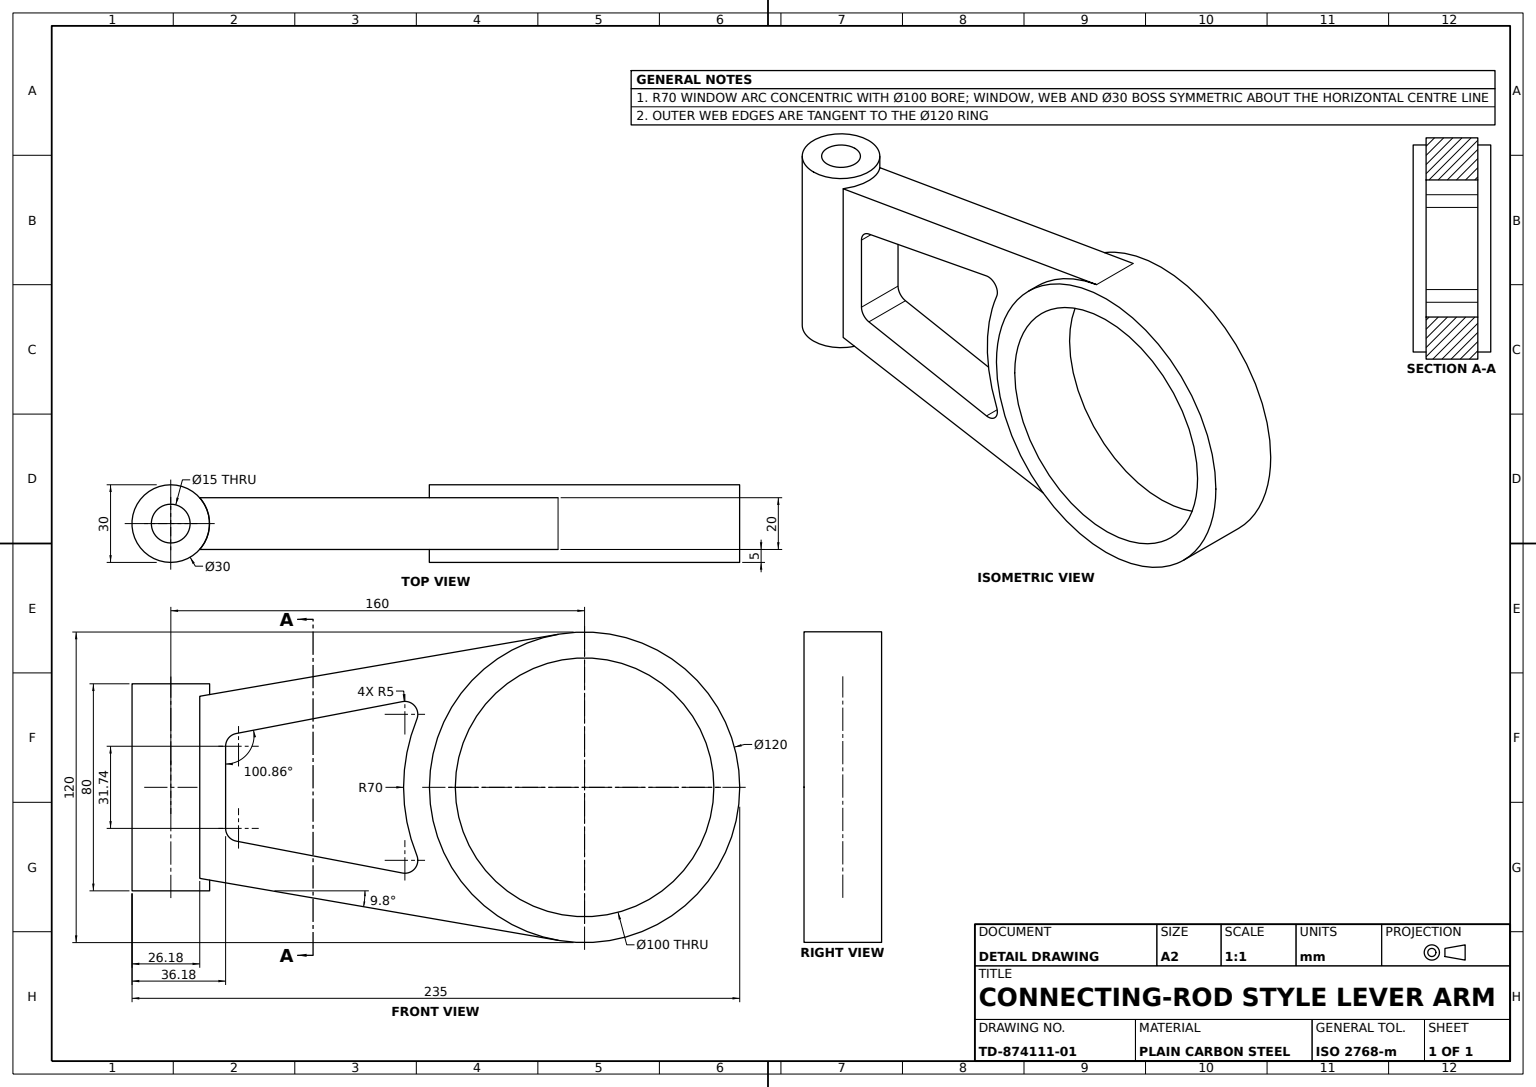
SolidWorks part; units mm, degrees
material "Plain Carbon Steel"
ref_plane "Front Plane" through (0, 0, 0) normal (0, 0, 1) x (1, 0, 0)
ref_plane "Top Plane" through (0, 0, 0) normal (0, 1, 0) x (1, 0, 0)
ref_plane "Right Plane" through (0, 0, 0) normal (1, 0, 0) x (0, 0, -1)
sketch "Big End Ring Sketch" plane through (0, 0, 0) normal (0, 0, 1) x (1, 0, 0)
  line L0 (-225.0888, 0) -> (225.0888, 0) construction
  line L1 (0, 149.419) -> (0, -149.419) construction
  circle A0 centre (0, 0) radius 50
  circle A1 centre (0, 0) radius 60
  point P4 (0, 0)
  point P8 (0, 0)
  dimension "D1" = 120
  dimension "D2" = 100
extrude "Big End Ring Ø120" add sketch "Big End Ring Sketch" along normal mid plane 30
sketch "Small End Boss Sketch" plane through (0, 0, 0) normal (0, 1, 0) x (1, 0, 0)
  line L0 (0, 62.5655) -> (0, -62.5655) construction
  circle A0 centre (-160, 0) radius 7.5
  circle A1 centre (-160, 0) radius 15
  point P4 (0, 0)
  dimension "D1" = 30
  dimension "D2" = 15
  dimension "D3" = 160
extrude "Small End Boss Ø30" add sketch "Small End Boss Sketch" along normal mid plane 80 separate body
sketch "Web Profile Sketch" plane through (0, 0, 0) normal (0, 0, 1) x (1, 0, 0)
  line L0 (-10.2129, 59.1244) -> (-149.8732, 35)
  line L1 (-10.2129, -59.1244) -> (-149.8732, -35)
  line L2 (-149.8732, 35) -> (-149.8732, -35)
  line L3 (268.3602, 0) -> (-268.3602, 0) construction
  line L4 (-126.6407, 20) -> (-126.6407, -20)
  line L5 (-70.7566, 32.6973) -> (-126.6407, 20)
  line L6 (-126.6407, -20) -> (-70.7566, -32.6973)
  circle A0 centre (0, 0) radius 60 construction
  arc A1 (-10.2129, 59.1244) -> (-10.2129, -59.1244) centre (0, 0) ccw
  arc A2 (-65.0056, 25.9668) -> (-65.0056, -25.9668) centre (0, 0) ccw
  arc A3 (-65.0056, -25.9668) -> (-70.7566, -32.6973) centre (-69.6488, -27.8215) cw
  arc A4 (-65.0056, 25.9668) -> (-70.7566, 32.6973) centre (-69.6488, 27.8215) ccw
  point P10 (0, 0)
  point P15 (-60.6218, -35)
  point P18 (-60.6218, 35)
  dimension "D1" = 140
  dimension "D4" = 5
  dimension "D2" = 70
  dimension "D3" = 35
  dimension "D5" = 40
  dimension "D6" = 20
  dimension "D7" = 70
  dimension "D8" = 35
  dimension "D9" = 149.8732
  dimension "D10" = 126.6407
extrude "Connecting Web" add sketch "Web Profile Sketch" along normal mid plane 20 contours L0 L2 L1 A1
sketch "Web Window Sketch" plane through (0, 0, 10) normal (0, 0, 1) x (1, 0, 0)
  line L0 (189.2397, 0) -> (-189.2397, 0) construction
  line L1 (-138.8197, 15.8679) -> (-138.8197, -15.8679)
  line L2 (-134.7616, 20.7784) -> (-70.4356, 33.1175)
  line L3 (-134.7616, -20.7784) -> (-70.4356, -33.1175)
  line L4 (-148.8197, 35.182) -> (-148.8197, -35.182) construction
  arc A1 (-64.8607, 26.3266) -> (-64.8607, -26.3266) centre (0, 0) ccw
  arc A2 (-134.7616, 20.7784) -> (-138.8197, 15.8679) centre (-133.8197, 15.8679) ccw
  arc A3 (-134.7616, -20.7784) -> (-138.8197, -15.8679) centre (-133.8197, -15.8679) cw
  arc A4 (-70.4356, -33.1175) -> (-64.8607, -26.3266) centre (-69.4936, -28.207) ccw
  arc A5 (-64.8607, 26.3266) -> (-70.4356, 33.1175) centre (-69.4936, 28.207) ccw
  point P6 (0, 0)
  point P11 (-138.8197, 20)
  point P14 (-138.8197, -20)
  point P17 (-60.6218, -35)
  point P20 (-60.6218, 35)
  point P23 (-138.8197, 0)
  dimension "D1" = 70
  dimension "D6" = 5
  dimension "D2" = 20
  dimension "D3" = 20
  dimension "D4" = 70
  dimension "D5" = 35
  dimension "D7" = 10
extrude "Web Lightening Window" cut sketch "Web Window Sketch" against normal mid plane 105
